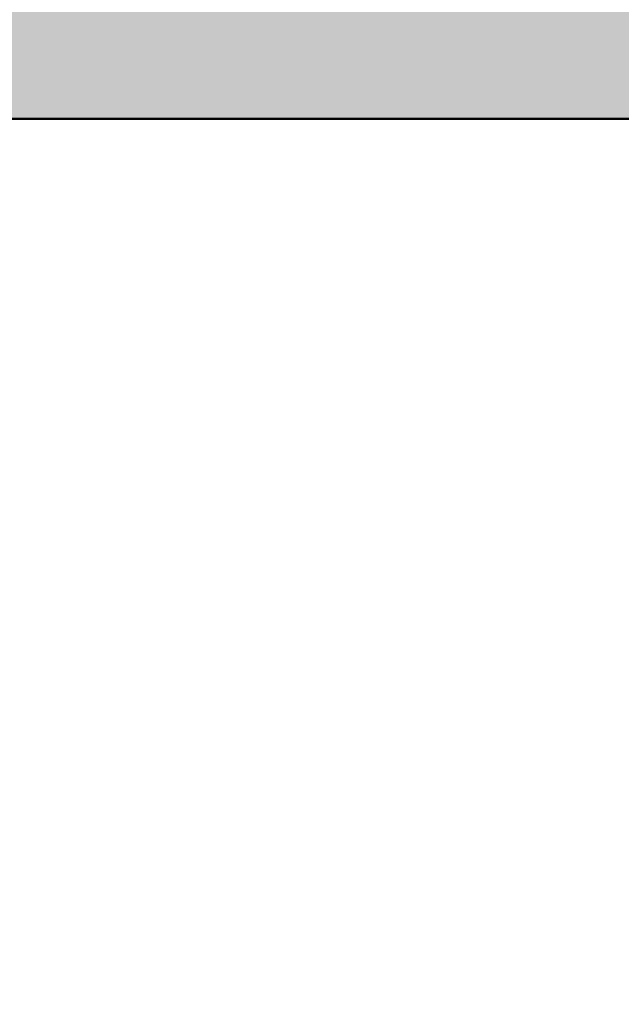
# Model space of a CAD drawing. Units: inches. Extents: x 22042254 to 25404563, y 17568978 to 17626777.
# Tile 35 of 45: x 22179890 to 22179932, y 17626332 to 17626402. Entities that reach past the tile are written whole.
import ezdxf

# ---------------------------------------------------------------- set-up
doc = ezdxf.new("R2010")
doc.units = ezdxf.units.IN
doc.header["$MEASUREMENT"] = 0
doc.layers.add('A-WALL-PATT', color=244, linetype='Continuous', lineweight=13)
doc.layers.add('walls', color=252, linetype='Continuous', lineweight=50)

msp = doc.modelspace()

# ---------------------------------------------------------------- hatches: boundary and pattern name
at = {"layer": 'A-WALL-PATT'}
h = msp.add_hatch(color=256, dxfattribs=at)
h.dxf.hatch_style = 1
h.paths.add_polyline_path([(22179792.734, 17626580.28), (22179888.734, 17626580.28), (22179888.734, 17626559.623), (22179893.234, 17626559.623), (22179893.234, 17626580.28), (22179900.438, 17626580.28), (22179900.438, 17626584.78), (22179792.734, 17626584.78), (22179792.734, 17626728.78), (22180134.734, 17626728.78), (22180134.734, 17626584.78), (22180035.602, 17626584.78), (22180004.432, 17626584.78), (22180001.734, 17626584.78), (22180001.734, 17626580.28), (22180134.734, 17626580.28), (22180134.734, 17626404.28), (22180064.487, 17626404.28), (22180064.487, 17626399.78), (22180134.734, 17626399.78), (22180134.734, 17626197.78), (22180143.734, 17626197.78), (22180143.734, 17626737.78), (22179783.734, 17626737.78), (22179783.734, 17626197.78), (22179792.734, 17626197.78), (22179792.734, 17626394.78), (22179936.734, 17626394.78), (22179936.734, 17626383.208), (22179941.234, 17626383.208), (22179941.234, 17626532.28), (22179927.066, 17626532.28), (22179927.066, 17626527.78), (22179928.072, 17626527.78), (22179936.734, 17626527.78), (22179936.734, 17626403.78), (22179792.734, 17626403.78), (22179792.734, 17626527.78), (22179905.094, 17626527.78), (22179905.094, 17626532.28), (22179792.734, 17626532.28)])

# ---------------------------------------------------------------- linework, layer by layer
at = {"layer": 'walls'}
msp.add_line((22179792.734, 17626394.78), (22179936.734, 17626394.78), dxfattribs=at)

doc.saveas('drawing.dxf')
